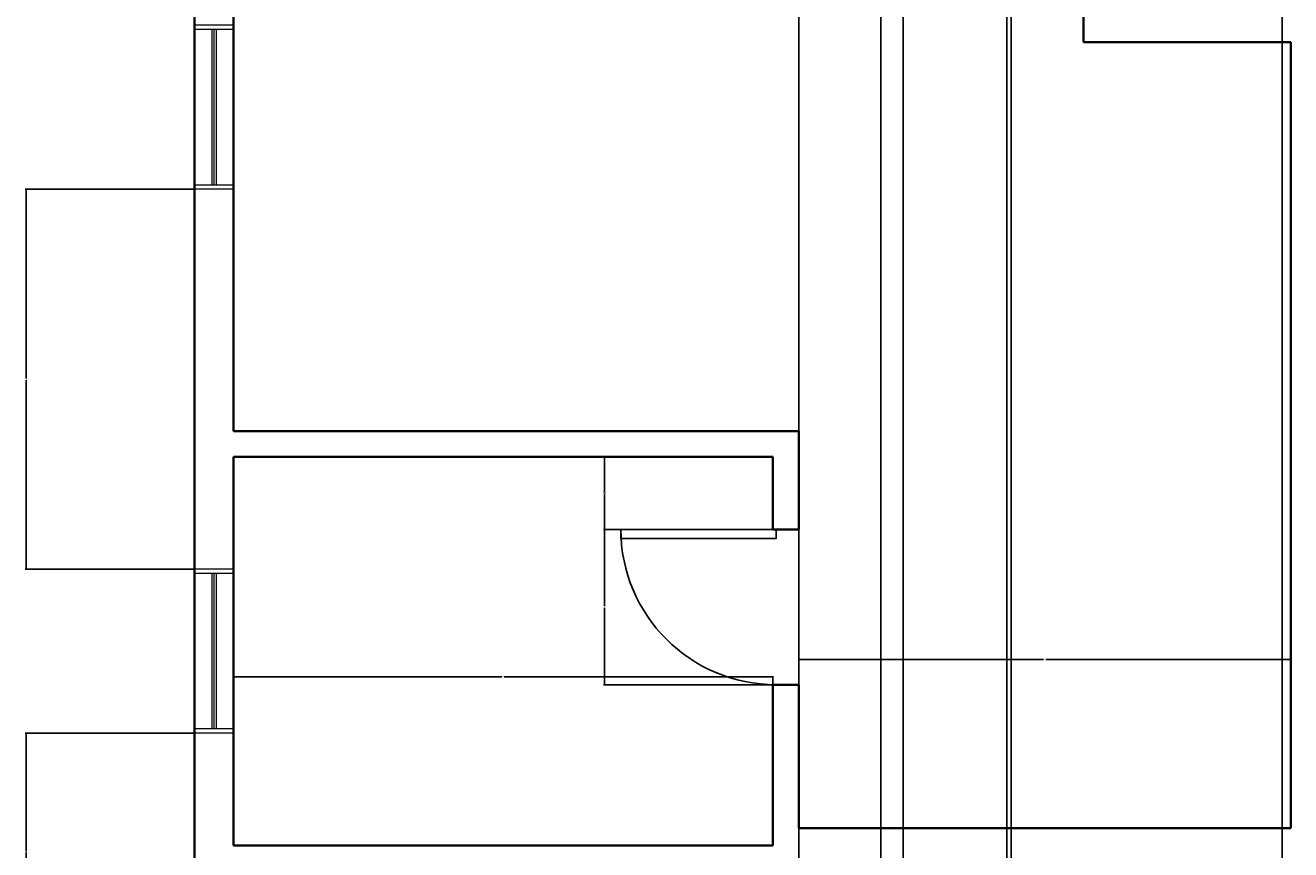
# Model space of a CAD drawing. Units: inches. Extents: x -7288 to -6705, y 7169 to 8028.
# Tile 3 of 5: x -7288 to -6995, y 7493 to 7684. Entities that reach past the tile are written whole.
import ezdxf

# ---------------------------------------------------------------- set-up
doc = ezdxf.new("R2010")
doc.units = ezdxf.units.IN
for name, color, linetype, lineweight in [('A-ANNO-DIMS', 2, 'Continuous', 18), ('A-DOOR', 3, 'Continuous', 25), ('A-GLAZ', 2, 'Continuous', 18), ('A-WALL', 1, 'Continuous', 35)]:
    doc.layers.add(name, color=color, linetype=linetype, lineweight=lineweight)
doc.styles.get("Standard").update_dxf_attribs({"font": 'arial.ttf'})
doc.dimstyles.get("Standard").update_dxf_attribs({"dimtxt": 0.18, "dimasz": 0.18, "dimexe": 0.18, "dimexo": 0.0625, "dimgap": 0.09, "dimtad": 0, "dimtih": 1, "dimtoh": 1, "dimdec": 4, "dimzin": 0, "dimdsep": 46, "dimtxsty": 'Standard', "dimcen": 0.09, "dimadec": 0, "dimazin": 0, "dimtfac": 1, "dimtdec": 4, "dimtofl": 0, "dimtmove": 0, "dimatfit": 3, "dimfxl": 1, "dimtolj": 1, "dimtzin": 0, "dimarcsym": 0})

# ---------------------------------------------------------------- blocks, each defined once
blk = doc.blocks.new('*U8')
for p, q in [((0, 0), (0, -100)), ((750, 0), (750, -100))]:
    blk.add_line(p, q)
blk.add_lwpolyline([(0, 0), (0, 750), (43.75, 750), (43.75, 0)], close=True)
blk.add_arc((0, 0), 750, 0, 90)
blk = doc.blocks.new('WIN-36IN-WALL9')
for p, q in [((0, 38), (9, 38)), ((0, 37), (9, 37)), ((4, 1), (4, 37)), ((4.5, 1), (4.5, 37)), ((5, 1), (5, 37)), ((0, 1), (9, 1)), ((0, 0), (9, 0))]:
    blk.add_line(p, q)
blk = doc.blocks.new('*D103')
at = {"layer": 'A-ANNO-DIMS', "color": 0, "lineweight": -2, "transparency": 16777216}
for p, q in [((-7089.84, 7838.47), (-7089.84, 7169.32)), ((-6996.84, 7838.47), (-6996.84, 7169.32)), ((-7089.66, 7169.5), (-7043.56, 7169.5)), ((-6997.02, 7169.5), (-7043.12, 7169.5))]:
    blk.add_line(p, q, dxfattribs=at)
at = {"layer": 'A-ANNO-DIMS', "color": 0, "transparency": 16777216}
for points in [[(-7089.66, 7169.53), (-7089.66, 7169.47), (-7089.84, 7169.5)], [(-6997.02, 7169.53), (-6997.02, 7169.47), (-6996.84, 7169.5)]]:
    blk.add_solid(points, dxfattribs=at)
at = {"layer": 'Defpoints', "color": 0, "transparency": 16777216}
for p in [(-7089.84, 7838.53), (-6996.84, 7838.53), (-6996.84, 7169.5)]:
    blk.add_point(p, dxfattribs=at)
at = {"layer": 'A-ANNO-DIMS', "color": 0, "transparency": 16777216, "insert": (-7043.34, 7169.5), "char_height": 0.18, "attachment_point": 5}
blk.add_mtext('\\A1;93', dxfattribs=at)
blk = doc.blocks.new('*D119')
at = {"layer": 'A-ANNO-DIMS', "color": 0, "lineweight": -2, "transparency": 16777216}
for p, q in [((-7089.84, 7799.47), (-7089.84, 7169.32)), ((-7059.61, 7799.47), (-7059.61, 7169.32)), ((-7089.66, 7169.5), (-7075.12, 7169.5)), ((-7059.79, 7169.5), (-7074.33, 7169.5))]:
    blk.add_line(p, q, dxfattribs=at)
at = {"layer": 'A-ANNO-DIMS', "color": 0, "transparency": 16777216}
for points in [[(-7089.66, 7169.53), (-7089.66, 7169.47), (-7089.84, 7169.5)], [(-7059.79, 7169.53), (-7059.79, 7169.47), (-7059.61, 7169.5)]]:
    blk.add_solid(points, dxfattribs=at)
at = {"layer": 'Defpoints', "color": 0, "transparency": 16777216}
for p in [(-7089.84, 7799.53), (-7059.61, 7799.53), (-7059.61, 7169.5)]:
    blk.add_point(p, dxfattribs=at)
at = {"layer": 'A-ANNO-DIMS', "color": 0, "transparency": 16777216, "insert": (-7074.72, 7169.5), "char_height": 0.18, "attachment_point": 5}
blk.add_mtext('\\A1;30.23', dxfattribs=at)
blk = doc.blocks.new('*D131')
at = {"layer": 'A-ANNO-DIMS', "color": 0, "lineweight": -2, "transparency": 16777216}
for p, q in [((-7108.84, 7497.59), (-7108.84, 7536.74)), ((-7108.66, 7536.56), (-7052.12, 7536.56)), ((-6995.02, 7536.56), (-7051.56, 7536.56)), ((-6994.84, 7497.59), (-6994.84, 7536.74))]:
    blk.add_line(p, q, dxfattribs=at)
at = {"layer": 'A-ANNO-DIMS', "color": 0, "transparency": 16777216}
for points in [[(-7108.66, 7536.59), (-7108.66, 7536.53), (-7108.84, 7536.56)], [(-6995.02, 7536.59), (-6995.02, 7536.53), (-6994.84, 7536.56)]]:
    blk.add_solid(points, dxfattribs=at)
at = {"layer": 'Defpoints', "color": 0, "transparency": 16777216}
for p in [(-6994.84, 7536.56), (-7108.84, 7497.53), (-6994.84, 7497.53)]:
    blk.add_point(p, dxfattribs=at)
at = {"layer": 'A-ANNO-DIMS', "color": 0, "transparency": 16777216, "insert": (-7051.84, 7536.56), "char_height": 0.18, "attachment_point": 5}
blk.add_mtext('\\A1;114', dxfattribs=at)
blk = doc.blocks.new('*D137')
at = {"layer": 'A-ANNO-DIMS', "color": 0, "lineweight": -2, "transparency": 16777216}
for p, q in [((-7239.84, 7493.59), (-7239.84, 7532.74)), ((-7114.84, 7493.59), (-7114.84, 7532.74)), ((-7239.66, 7532.56), (-7177.62, 7532.56)), ((-7115.02, 7532.56), (-7177.06, 7532.56))]:
    blk.add_line(p, q, dxfattribs=at)
at = {"layer": 'A-ANNO-DIMS', "color": 0, "transparency": 16777216}
for points in [[(-7239.66, 7532.59), (-7239.66, 7532.53), (-7239.84, 7532.56)], [(-7115.02, 7532.59), (-7115.02, 7532.53), (-7114.84, 7532.56)]]:
    blk.add_solid(points, dxfattribs=at)
at = {"layer": 'Defpoints', "color": 0, "transparency": 16777216}
for p in [(-7114.84, 7532.56), (-7239.84, 7493.53), (-7114.84, 7493.53)]:
    blk.add_point(p, dxfattribs=at)
at = {"layer": 'A-ANNO-DIMS', "color": 0, "transparency": 16777216, "insert": (-7177.34, 7532.56), "char_height": 0.18, "attachment_point": 5}
blk.add_mtext('\\A1;125', dxfattribs=at)
blk = doc.blocks.new('*D148')
at = {"layer": 'A-ANNO-DIMS', "color": 0, "lineweight": -2, "transparency": 16777216}
for p, q in [((-7248.9, 7519.53), (-7288.05, 7519.53)), ((-7287.87, 7519.35), (-7287.87, 7492.21)), ((-7287.87, 7464.71), (-7287.87, 7491.85)), ((-7248.9, 7464.53), (-7288.05, 7464.53))]:
    blk.add_line(p, q, dxfattribs=at)
at = {"layer": 'A-ANNO-DIMS', "color": 0, "transparency": 16777216}
for points in [[(-7287.9, 7519.35), (-7287.84, 7519.35), (-7287.87, 7519.53)], [(-7287.9, 7464.71), (-7287.84, 7464.71), (-7287.87, 7464.53)]]:
    blk.add_solid(points, dxfattribs=at)
at = {"layer": 'Defpoints', "color": 0, "transparency": 16777216}
for p in [(-7287.87, 7519.53), (-7248.84, 7519.53), (-7248.84, 7464.53)]:
    blk.add_point(p, dxfattribs=at)
at = {"layer": 'A-ANNO-DIMS', "color": 0, "transparency": 16777216, "insert": (-7287.87, 7492.03), "char_height": 0.18, "attachment_point": 5}
blk.add_mtext('\\A1;55', dxfattribs=at)
blk = doc.blocks.new('*D149')
at = {"layer": 'A-ANNO-DIMS', "color": 0, "lineweight": -2, "transparency": 16777216}
for p, q in [((-7248.9, 7645.53), (-7288.05, 7645.53)), ((-7287.87, 7645.35), (-7287.87, 7601.71)), ((-7287.87, 7557.71), (-7287.87, 7601.35)), ((-7248.9, 7557.53), (-7288.05, 7557.53))]:
    blk.add_line(p, q, dxfattribs=at)
at = {"layer": 'A-ANNO-DIMS', "color": 0, "transparency": 16777216}
for points in [[(-7287.9, 7645.35), (-7287.84, 7645.35), (-7287.87, 7645.53)], [(-7287.9, 7557.71), (-7287.84, 7557.71), (-7287.87, 7557.53)]]:
    blk.add_solid(points, dxfattribs=at)
at = {"layer": 'Defpoints', "color": 0, "transparency": 16777216}
for p in [(-7287.87, 7645.53), (-7248.84, 7645.53), (-7248.84, 7557.53)]:
    blk.add_point(p, dxfattribs=at)
at = {"layer": 'A-ANNO-DIMS', "color": 0, "transparency": 16777216, "insert": (-7287.87, 7601.53), "char_height": 0.18, "attachment_point": 5}
blk.add_mtext('\\A1;88', dxfattribs=at)
blk = doc.blocks.new('*D156')
at = {"layer": 'A-ANNO-DIMS', "color": 0, "lineweight": -2, "transparency": 16777216}
for p, q in [((-7084.64, 7347.59), (-7084.64, 8027.74)), ((-7084.46, 8027.56), (-7072.86, 8027.56)), ((-7060.82, 8027.56), (-7072.42, 8027.56)), ((-7060.64, 7347.59), (-7060.64, 8027.74))]:
    blk.add_line(p, q, dxfattribs=at)
at = {"layer": 'A-ANNO-DIMS', "color": 0, "transparency": 16777216}
for points in [[(-7084.46, 8027.59), (-7084.46, 8027.53), (-7084.64, 8027.56)], [(-7060.82, 8027.59), (-7060.82, 8027.53), (-7060.64, 8027.56)]]:
    blk.add_solid(points, dxfattribs=at)
at = {"layer": 'Defpoints', "color": 0, "transparency": 16777216}
for p in [(-7060.64, 8027.56), (-7084.64, 7347.53), (-7060.64, 7347.53)]:
    blk.add_point(p, dxfattribs=at)
at = {"layer": 'A-ANNO-DIMS', "color": 0, "transparency": 16777216, "insert": (-7072.64, 8027.56), "char_height": 0.18, "attachment_point": 5}
blk.add_mtext('\\A1;24', dxfattribs=at)
blk = doc.blocks.new('*D157')
at = {"layer": 'A-ANNO-DIMS', "color": 0, "lineweight": -2, "transparency": 16777216}
for p, q in [((-7108.84, 7347.59), (-7108.84, 8027.74)), ((-7108.66, 8027.56), (-7097.07, 8027.56)), ((-7084.82, 8027.56), (-7096.42, 8027.56)), ((-7084.64, 7347.59), (-7084.64, 8027.74))]:
    blk.add_line(p, q, dxfattribs=at)
at = {"layer": 'A-ANNO-DIMS', "color": 0, "transparency": 16777216}
for points in [[(-7108.66, 8027.59), (-7108.66, 8027.53), (-7108.84, 8027.56)], [(-7084.82, 8027.59), (-7084.82, 8027.53), (-7084.64, 8027.56)]]:
    blk.add_solid(points, dxfattribs=at)
at = {"layer": 'Defpoints', "color": 0, "transparency": 16777216}
for p in [(-7084.64, 8027.56), (-7108.84, 7347.53), (-7084.64, 7347.53)]:
    blk.add_point(p, dxfattribs=at)
at = {"layer": 'A-ANNO-DIMS', "color": 0, "transparency": 16777216, "insert": (-7096.74, 8027.56), "char_height": 0.18, "attachment_point": 5}
blk.add_mtext('\\A1;24.2', dxfattribs=at)
blk = doc.blocks.new('*D164')
at = {"layer": 'A-ANNO-DIMS', "color": 0, "lineweight": -2, "transparency": 16777216}
for p, q in [((-7114.9, 7566.74), (-7154.05, 7566.74)), ((-7153.87, 7566.56), (-7153.87, 7548.93)), ((-7153.87, 7530.92), (-7153.87, 7548.56)), ((-7114.9, 7530.74), (-7154.05, 7530.74))]:
    blk.add_line(p, q, dxfattribs=at)
at = {"layer": 'A-ANNO-DIMS', "color": 0, "transparency": 16777216}
for points in [[(-7153.9, 7566.56), (-7153.84, 7566.56), (-7153.87, 7566.74)], [(-7153.9, 7530.92), (-7153.84, 7530.92), (-7153.87, 7530.74)]]:
    blk.add_solid(points, dxfattribs=at)
at = {"layer": 'Defpoints', "color": 0, "transparency": 16777216}
for p in [(-7153.87, 7566.74), (-7114.84, 7566.74), (-7114.84, 7530.74)]:
    blk.add_point(p, dxfattribs=at)
at = {"layer": 'A-ANNO-DIMS', "color": 0, "transparency": 16777216, "insert": (-7153.87, 7548.74), "char_height": 0.18, "attachment_point": 5}
blk.add_mtext('\\A1;36', dxfattribs=at)
blk = doc.blocks.new('*D165')
at = {"layer": 'A-ANNO-DIMS', "color": 0, "lineweight": -2, "transparency": 16777216}
for p, q in [((-7114.9, 7583.53), (-7154.05, 7583.53)), ((-7153.87, 7583.35), (-7153.87, 7575.32)), ((-7153.87, 7566.92), (-7153.87, 7574.96)), ((-7114.9, 7566.74), (-7154.05, 7566.74))]:
    blk.add_line(p, q, dxfattribs=at)
at = {"layer": 'A-ANNO-DIMS', "color": 0, "transparency": 16777216}
for points in [[(-7153.9, 7583.35), (-7153.84, 7583.35), (-7153.87, 7583.53)], [(-7153.9, 7566.92), (-7153.84, 7566.92), (-7153.87, 7566.74)]]:
    blk.add_solid(points, dxfattribs=at)
at = {"layer": 'Defpoints', "color": 0, "transparency": 16777216}
for p in [(-7153.87, 7583.53), (-7114.84, 7583.53), (-7114.84, 7566.74)]:
    blk.add_point(p, dxfattribs=at)
at = {"layer": 'A-ANNO-DIMS', "color": 0, "transparency": 16777216, "insert": (-7153.87, 7575.14), "char_height": 0.18, "attachment_point": 5}
blk.add_mtext('\\A1;16.787', dxfattribs=at)

msp = doc.modelspace()

# ---------------------------------------------------------------- linework, layer by layer
at = {"layer": 'A-WALL'}
for p, q in [((-7248.8398, 7208.5311), (-7248.8398, 7958.5311)), ((-7239.8398, 7589.5311), (-7239.8398, 7739.5311)), ((-7042.8398, 7685.639), (-7042.8398, 7679.639)), ((-7042.8398, 7679.639), (-6994.8398, 7679.639)), ((-6994.8398, 7497.5311), (-6994.8398, 7679.639)), ((-7239.8398, 7589.5311), (-7108.8398, 7589.5311)), ((-7108.8398, 7566.7444), (-7108.8398, 7589.5311)), ((-7239.8398, 7583.5311), (-7114.8398, 7583.5311)), ((-7239.8398, 7493.5311), (-7239.8398, 7583.5311)), ((-7114.8398, 7566.7444), (-7114.8398, 7583.5311)), ((-7114.8398, 7566.7444), (-7108.8398, 7566.7444)), ((-7114.8398, 7493.5311), (-7114.8398, 7530.7444)), ((-7114.8398, 7530.7444), (-7108.8398, 7530.7444)), ((-7108.8398, 7497.5311), (-7108.8398, 7530.7444)), ((-6994.8398, 7497.5311), (-7108.8398, 7497.5311)), ((-7239.8398, 7493.5311), (-7114.8398, 7493.5311))]:
    msp.add_line(p, q, dxfattribs=at)

# ---------------------------------------------------------------- block references
at = {"layer": 'A-DOOR', "xscale": -0.0479970023277597, "yscale": 0.0479970023277597, "zscale": 0.0479970023277597, "rotation": 90}
msp.add_blockref('*U8', (-7114.0553, 7566.7421), dxfattribs=at)
at = {"layer": 'A-GLAZ', "rotation": 180}
for p in [(-7239.8398, 7683.5311), (-7239.8398, 7557.5311)]:
    msp.add_blockref('WIN-36IN-WALL9', p, dxfattribs=at)

# ---------------------------------------------------------------- dimensions: what is measured, and where the dimension line sits
at = {"layer": 'A-ANNO-DIMS'}
for base, p1, p2, override, picture, middle in [((-7084.6414, 8027.5611), (-7108.8398, 7347.5311), (-7084.6414, 7347.5311), {"dimdec": 1, "dimlfac": 1, "dimrnd": 0, "dimzin": 0, "dimdsep": 46, "dimlunit": 2}, '*D157', (-7096.7406, 8027.5611)), ((-7060.6414, 8027.5611), (-7084.6414, 7347.5311), (-7060.6414, 7347.5311), {"dimdec": 0, "dimlfac": 1, "dimrnd": 0, "dimzin": 0, "dimdsep": 46, "dimlunit": 2}, '*D156', (-7072.6414, 8027.5611)), ((-6996.8398, 7169.5011), (-7089.8398, 7838.5311), (-6996.8398, 7838.5311), {"dimdec": 0, "dimlfac": 1, "dimrnd": 0, "dimzin": 0, "dimdsep": 46, "dimlunit": 2}, '*D103', (-7043.3398, 7169.5011)), ((-7059.607, 7169.5011), (-7089.8398, 7799.5311), (-7059.607, 7799.5311), {"dimdec": 2, "dimlfac": 1, "dimrnd": 0, "dimzin": 0, "dimdsep": 46, "dimlunit": 2}, '*D119', (-7074.7234, 7169.5011)), ((-6994.8398, 7536.5611), (-7108.8398, 7497.5311), (-6994.8398, 7497.5311), {"dimdec": 0, "dimlfac": 1, "dimrnd": 0, "dimzin": 0, "dimdsep": 46, "dimlunit": 2}, '*D131', (-7051.8398, 7536.5611)), ((-7114.8398, 7532.5611), (-7239.8398, 7493.5311), (-7114.8398, 7493.5311), {"dimdec": 0, "dimlfac": 1, "dimrnd": 0, "dimzin": 0, "dimdsep": 46, "dimlunit": 2}, '*D137', (-7177.3398, 7532.5611))]:
    dim = msp.add_linear_dim(base=base, p1=p1, p2=p2, dimstyle='Standard', override=override, dxfattribs=at)
    dim.commit()
    dim.dimension.update_dxf_attribs({"geometry": picture, "text_midpoint": middle})
for base, p1, p2, override, picture, middle in [((-7287.8698, 7645.5311), (-7248.8398, 7557.5311), (-7248.8398, 7645.5311), {"dimdec": 0, "dimlfac": 1, "dimrnd": 0, "dimzin": 0, "dimdsep": 46, "dimlunit": 2}, '*D149', (-7287.8698, 7601.5311)), ((-7153.8698, 7583.5311), (-7114.8398, 7566.7444), (-7114.8398, 7583.5311), {"dimdec": 3, "dimlfac": 1, "dimrnd": 0, "dimzin": 0, "dimdsep": 46, "dimlunit": 2}, '*D165', (-7153.8698, 7575.1377)), ((-7153.8698, 7566.7444), (-7114.8398, 7530.7444), (-7114.8398, 7566.7444), {"dimdec": 0, "dimlfac": 1, "dimrnd": 0, "dimzin": 0, "dimdsep": 46, "dimlunit": 2}, '*D164', (-7153.8698, 7548.7444)), ((-7287.8698, 7519.5311), (-7248.8398, 7464.5311), (-7248.8398, 7519.5311), {"dimdec": 0, "dimlfac": 1, "dimrnd": 0, "dimzin": 0, "dimdsep": 46, "dimlunit": 2}, '*D148', (-7287.8698, 7492.0311))]:
    dim = msp.add_linear_dim(base=base, p1=p1, p2=p2, angle=90, dimstyle='Standard', override=override, dxfattribs=at)
    dim.commit()
    dim.dimension.update_dxf_attribs({"geometry": picture, "text_midpoint": middle})

doc.saveas('drawing.dxf')
